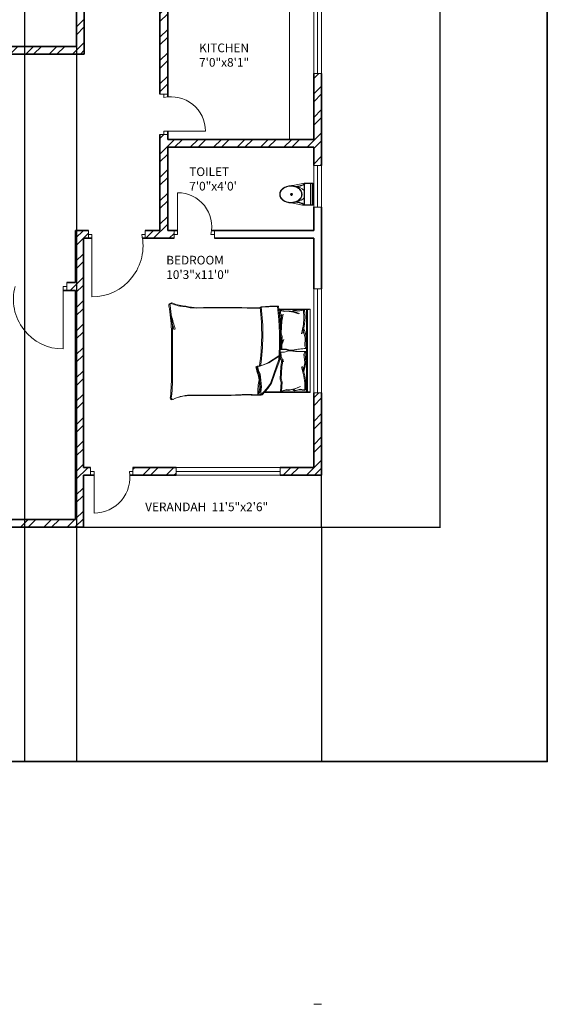
# Model space of a CAD drawing. Units: inches. Extents: x 1885 to 2748, y 783 to 2421.
# Tile 28 of 117: x 2445 to 2748, y 783 to 1350. Entities that reach past the tile are written whole.
import ezdxf

# ---------------------------------------------------------------- set-up
doc = ezdxf.new("R2010")
doc.units = ezdxf.units.IN
for name, color, linetype, lineweight in [('A-ANNO-DIMS', 2, 'Continuous', 18), ('A-ANNO-TTLB', 7, 'Continuous', 35), ('A-AREA-IDEN', 7, 'Continuous', 18), ('A-DOOR', 31, 'Continuous', 18), ('A-FLOR-BALC', 7, 'Continuous', 25), ('A-FLOR-CASE', 9, 'Continuous', 18), ('A-FLOR-FIXT', 8, 'Continuous', 18), ('A-FURN', 8, 'Continuous', 13), ('A-GENL-RVWE', 8, 'Continuous', 13), ('A-GLAZ', 181, 'Continuous', 18), ('A-WALL', 7, 'Continuous', 35)]:
    doc.layers.add(name, color=color, linetype=linetype, lineweight=lineweight)
doc.layers.add('A-WALL-PATT', color=85, linetype='Continuous', lineweight=13, true_color=0x58ba48)
doc.styles.get("Standard").update_dxf_attribs({"font": 'arial.ttf'})
doc.dimstyles.get("Standard").update_dxf_attribs({"dimtxt": 0.18, "dimasz": 0.18, "dimexe": 0.18, "dimexo": 0.0625, "dimgap": 0.09, "dimtad": 0, "dimtih": 1, "dimtoh": 1, "dimdec": 4, "dimzin": 0, "dimdsep": 46, "dimtxsty": 'Standard', "dimcen": 0.09, "dimadec": 0, "dimazin": 0, "dimtfac": 1, "dimtdec": 4, "dimtofl": 0, "dimtmove": 0, "dimatfit": 3, "dimfxl": 1, "dimtolj": 1, "dimtzin": 0, "dimarcsym": 0})

# ---------------------------------------------------------------- blocks, each defined once
blk = doc.blocks.new('A$C31115884')
for p, q in [((283, 498), (223, 498)), ((258, 466), (258, 523)), ((0, 200), (0, 0)), ((520, 200), (0, 200)), ((510, 54), (0, 54)), ((10, 190), (10, 10)), ((510, 190), (10, 190)), ((10, 10), (510, 10)), ((510, 10), (510, 190)), ((520, 0), (520, 200)), ((0, 0), (520, 0))]:
    blk.add_line(p, q)
blk.add_circle((256, 496), 23.6)
for centre, radius, start, end in [((2778, -205), 2807, 165.4549, 171.7133), ((-295, 403), 365, 324.2091, 9.3499), ((-295, 403), 375, 324.2091, 9.3499), ((806, 403), 365, 170.6501, 215.7909), ((3237, 905), 2807, 188.2867, 194.5451), ((384, 406), 293, 190.2774, 224.1564), ((139, 406), 293, 315.8436, 2.6563), ((806, 403), 375, 179.2036, 215.7909)]:
    blk.add_arc(centre, radius, start, end)
blk.add_ellipse((256, 510), major_axis=(0, -261), ratio=0.772727)
blk.add_open_spline([(256, 259), (263, 259), (270, 260), (288, 262), (299, 265), (320, 273), (330, 278), (350, 291), (360, 299), (378, 316), (386, 326), (402, 347), (409, 358), (421, 383), (427, 395), (436, 422), (440, 436), (445, 465), (447, 480), (448, 509), (448, 524), (445, 553), (443, 568), (436, 596), (432, 610), (422, 636), (416, 649), (402, 672), (395, 683), (379, 703), (370, 712), (351, 728), (341, 735), (321, 746), (310, 751), (289, 757), (278, 759), (256, 761), (245, 761), (223, 757), (212, 754), (191, 746), (181, 741), (161, 728), (151, 720), (133, 703), (125, 693), (110, 672), (103, 660), (90, 636), (85, 623), (76, 596), (72, 582), (67, 553), (66, 538), (64, 509), (65, 494), (68, 465), (70, 450), (77, 422), (81, 408), (91, 382), (97, 370), (111, 346), (118, 335), (135, 316), (144, 307), (162, 291), (172, 284), (193, 273), (203, 269), (225, 262), (236, 260), (250, 259), (253, 259), (256, 259)], degree=3, knots=[0, 0, 0, 0, 0.110105, 0.110105, 0.285049, 0.285049, 0.459994, 0.459994, 0.634938, 0.634938, 0.809882, 0.809882, 0.984827, 0.984827, 1.159771, 1.159771, 1.334715, 1.334715, 1.50966, 1.50966, 1.684604, 1.684604, 1.859549, 1.859549, 2.034493, 2.034493, 2.209437, 2.209437, 2.384382, 2.384382, 2.559326, 2.559326, 2.73427, 2.73427, 2.909215, 2.909215, 3.084159, 3.084159, 3.259103, 3.259103, 3.434048, 3.434048, 3.608992, 3.608992, 3.783936, 3.783936, 3.958881, 3.958881, 4.133825, 4.133825, 4.30877, 4.30877, 4.483714, 4.483714, 4.658658, 4.658658, 4.833603, 4.833603, 5.008547, 5.008547, 5.183491, 5.183491, 5.358436, 5.358436, 5.53338, 5.53338, 5.708324, 5.708324, 5.883269, 5.883269, 6.058213, 6.058213, 6.233158, 6.233158, 6.283185, 6.283185, 6.283185, 6.283185])
blk = doc.blocks.new('BED-DOUBLE')
for p, q in [((0, 51.49), (0.64, 51.49)), ((0, 3.47), (0, 51.49)), ((0, 51.26), (26.61, 51.26)), ((0, 51.26), (26.61, 51.26)), ((0.64, 51.49), (27.25, 51.49)), ((0.64, 51.49), (27.25, 51.49)), ((1.54, 3.47), (1.54, 51.26)), ((1.54, 3.47), (1.54, 51.26)), ((2.18, 3.7), (2.18, 51.49)), ((2.18, 3.7), (2.18, 51.49)), ((27.75, 52.87), (24.5, 49.16)), ((27.75, 52.87), (24.5, 49.16)), ((28.39, 53.09), (25.14, 49.39)), ((28.39, 53.09), (25.14, 49.39)), ((29.49, 52.95), (27.75, 52.87, 3.87)), ((29.49, 52.95), (27.75, 52.87, 3.87)), ((28.37, 51.33), (27.75, 52.87)), ((28.37, 51.33), (27.75, 52.87)), ((28.06, 48.23), (28.37, 51.33)), ((28.06, 48.23), (28.37, 51.33)), ((30.13, 53.17), (28.39, 53.09, 3.87)), ((30.13, 53.17), (28.39, 53.09, 3.87)), ((29.01, 51.56), (28.39, 53.09)), ((29.01, 51.56), (28.39, 53.09)), ((28.7, 48.46), (29.01, 51.56)), ((28.7, 48.46), (29.01, 51.56)), ((2.56, 50.11), (2.46, 44.71)), ((2.56, 50.11), (2.46, 44.71)), ((2.46, 44.71), (2.55, 45.71)), ((2.46, 44.71), (2.55, 45.71)), ((2.55, 45.71), (3.07, 41.91)), ((2.55, 45.71), (3.07, 41.91)), ((2.56, 50.11), (5.77, 49.73)), ((2.56, 50.11), (5.77, 49.73)), ((3.2, 50.34), (3.1, 44.94)), ((3.2, 50.34), (3.1, 44.94)), ((3.1, 44.94), (3.19, 45.94)), ((3.1, 44.94), (3.19, 45.94)), ((3.19, 45.94), (3.71, 42.14)), ((3.19, 45.94), (3.71, 42.14)), ((3.2, 50.34), (6.41, 49.96)), ((3.2, 50.34), (6.41, 49.96)), ((8.26, 49.31), (5.58, 48.13)), ((8.26, 49.31), (5.58, 48.13)), ((5.77, 49.73), (8.34, 50.33)), ((5.77, 49.73), (8.34, 50.33)), ((8.9, 49.54), (6.22, 48.36)), ((8.9, 49.54), (6.22, 48.36)), ((6.41, 49.96), (8.98, 50.56)), ((6.41, 49.96), (8.98, 50.56)), ((11.83, 50.11), (8.26, 49.31)), ((11.83, 50.11), (8.26, 49.31)), ((8.34, 50.33), (9.39, 49.81)), ((8.34, 50.33), (9.39, 49.81)), ((12.47, 50.34), (8.9, 49.54)), ((12.47, 50.34), (8.9, 49.54)), ((8.98, 50.56), (10.03, 50.04)), ((8.98, 50.56), (10.03, 50.04)), ((13.44, 49.92), (11.83, 50.11)), ((13.44, 49.92), (11.83, 50.11)), ((14.08, 50.15), (12.47, 50.34)), ((14.08, 50.15), (12.47, 50.34)), ((16.58, 50.7), (13.44, 49.92)), ((16.58, 50.7), (13.44, 49.92)), ((17.22, 50.93), (14.08, 50.15)), ((17.22, 50.93), (14.08, 50.15)), ((16.17, 45.57), (16.58, 50.7)), ((16.17, 45.56), (16.58, 50.7)), ((16.73, 43.6), (16.17, 45.57)), ((16.73, 43.6), (16.17, 45.56)), ((16.81, 45.79), (17.22, 50.93)), ((16.81, 45.79), (17.22, 50.93)), ((17.37, 43.83), (16.81, 45.79)), ((17.37, 43.83), (16.81, 45.79)), ((22.33, 46.22), (20.32, 40.64)), ((22.33, 46.22), (20.32, 40.64)), ((22.97, 46.45), (20.96, 40.87)), ((22.97, 46.45), (20.96, 40.87)), ((24.5, 49.16), (22.33, 46.22)), ((24.5, 49.16), (22.33, 46.22)), ((25.14, 49.39), (22.97, 46.45)), ((25.14, 49.39), (22.97, 46.45)), ((28.37, 44.36), (28.06, 48.23)), ((28.37, 44.36), (28.06, 48.23)), ((29.01, 44.59), (28.7, 48.46)), ((29.01, 44.59), (28.7, 48.46)), ((3.07, 41.91), (4.43, 36.49)), ((3.07, 41.91), (4.43, 36.49)), ((3.71, 42.14), (5.07, 36.72)), ((3.71, 42.14), (5.07, 36.72)), ((16.3, 36.59), (16.73, 43.6)), ((16.3, 36.59), (16.73, 43.6)), ((16.94, 36.82), (17.37, 43.83)), ((16.94, 36.82), (17.37, 43.83)), ((20.32, 40.64), (17.39, 32.3)), ((20.32, 40.64), (17.39, 32.3)), ((20.96, 40.87), (18.03, 32.53)), ((20.96, 40.87), (18.03, 32.53)), ((28.83, 40.95), (28.37, 44.36)), ((28.83, 40.95), (28.37, 44.36)), ((29.76, 38.94), (28.83, 40.95)), ((29.76, 38.94), (28.83, 40.95)), ((29.47, 41.18), (29.01, 44.59)), ((29.47, 41.18), (29.01, 44.59)), ((30.4, 39.17), (29.47, 41.18)), ((30.4, 39.17), (29.47, 41.18)), ((79.89, 15.29), (79.89, 39.9)), ((79.89, 15.29), (79.89, 39.9)), ((3.08, 37.13), (2.54, 34.2)), ((3.08, 37.13), (2.54, 34.2)), ((2.54, 34.2), (2.56, 33.88)), ((2.54, 34.2), (2.56, 33.88)), ((3.68, 39.2), (3.08, 37.13)), ((3.68, 39.2), (3.08, 37.13)), ((3.72, 37.36), (3.18, 34.43)), ((3.72, 37.36), (3.18, 34.43)), ((3.18, 34.43), (3.2, 34.11)), ((3.18, 34.43), (3.2, 34.11)), ((3.2, 34.11), (3.62, 29.68)), ((3.2, 34.11), (3.62, 29.68)), ((4.32, 39.43), (3.72, 37.36)), ((4.32, 39.43), (3.72, 37.36)), ((15.63, 32.56), (16.3, 36.59)), ((15.63, 32.56), (16.3, 36.59)), ((17.38, 30.98), (16.1, 34.05)), ((17.38, 30.98), (16.1, 34.05)), ((16.27, 32.79), (16.94, 36.82)), ((16.27, 32.79), (16.94, 36.82)), ((17.39, 30.26), (23.88, 34.45)), ((17.39, 30.26), (23.88, 34.45)), ((18.03, 30.49), (24.52, 34.68)), ((18.03, 30.49), (24.52, 34.68)), ((23.88, 34.45), (28.37, 36.15)), ((23.88, 34.45), (28.37, 36.15)), ((24.52, 34.68), (29.01, 36.38)), ((24.52, 34.68), (29.01, 36.38)), ((28.37, 36.15), (30.38, 36.46)), ((28.37, 36.15), (30.38, 36.46)), ((29.01, 36.38), (31.02, 36.69)), ((29.01, 36.38), (31.02, 36.69)), ((30.38, 36.46), (29.76, 38.94)), ((30.38, 36.46), (29.76, 38.94)), ((31.02, 36.69), (30.4, 39.17)), ((31.02, 36.69), (30.4, 39.17)), ((79.25, 15.06), (79.25, 39.68)), ((79.25, 15.06), (79.25, 39.68)), ((2.98, 29.45), (2.5, 27.98)), ((2.98, 29.45), (2.5, 27.98)), ((2.56, 33.88), (2.98, 29.45)), ((2.56, 33.88), (2.98, 29.45)), ((3.62, 29.68), (3.13, 28.2)), ((3.62, 29.68), (3.13, 28.2)), ((14.86, 28.36), (17.54, 28.52)), ((14.86, 28.36), (17.54, 28.52)), ((16.74, 30.75), (15.46, 33.82)), ((16.74, 30.75), (15.46, 33.82)), ((16.9, 28.3), (16.74, 30.75)), ((16.9, 28.3), (16.74, 30.75)), ((17.54, 28.52), (17.38, 30.98)), ((17.54, 28.52), (17.38, 30.98)), ((1.87, 25.98), (7.22, 26.56)), ((1.87, 25.98), (7.22, 26.56)), ((2.45, 24.54), (1.87, 25.98)), ((2.45, 24.54), (1.87, 25.98)), ((2.31, 20.09), (2.45, 24.54)), ((2.31, 20.09), (2.45, 24.54)), ((2.5, 27.98), (7.87, 27.73)), ((2.5, 27.98), (7.87, 27.73)), ((2.51, 26.21), (7.86, 26.79)), ((2.51, 26.21), (7.86, 26.79)), ((3.09, 24.76), (2.51, 26.21)), ((3.09, 24.76), (2.51, 26.21)), ((2.95, 20.32), (3.09, 24.76)), ((2.95, 20.32), (3.09, 24.76)), ((3.13, 28.2), (8.51, 27.96)), ((3.13, 28.2), (8.51, 27.96)), ((7.22, 26.56), (10.4, 27.14)), ((7.22, 26.56), (10.4, 27.14)), ((7.86, 26.79), (11.04, 27.37)), ((7.86, 26.79), (11.04, 27.37)), ((7.87, 27.73), (11.08, 27.35)), ((7.87, 27.73), (11.08, 27.35)), ((8.51, 27.96), (11.72, 27.58)), ((8.51, 27.96), (11.72, 27.58)), ((10.4, 27.14), (11.71, 27.14)), ((10.4, 27.14), (11.71, 27.14)), ((11.04, 27.37), (12.35, 27.37)), ((11.04, 27.37), (12.35, 27.37)), ((11.08, 27.35), (12.38, 27.43)), ((11.08, 27.35), (12.38, 27.43)), ((11.71, 27.14), (13.59, 26.56)), ((11.71, 27.14), (13.59, 26.56)), ((11.72, 27.58), (13.02, 27.66)), ((11.72, 27.58), (13.02, 27.66)), ((12.35, 27.37), (14.22, 26.79)), ((12.35, 27.37), (14.22, 26.79)), ((12.38, 27.43), (14.22, 28.13)), ((12.38, 27.43), (14.22, 28.13)), ((13.02, 27.66), (14.86, 28.36)), ((13.02, 27.66), (14.86, 28.36)), ((13.59, 26.56), (16.27, 26.56)), ((13.59, 26.56), (16.27, 26.56)), ((14.22, 28.13), (16.9, 28.3)), ((14.22, 28.13), (16.9, 28.3)), ((14.22, 26.79), (16.91, 26.79)), ((14.22, 26.79), (16.91, 26.79)), ((16.27, 24.1), (15.18, 20.96)), ((16.27, 24.1), (15.18, 20.96)), ((16.91, 24.33), (15.82, 21.19)), ((16.91, 24.33), (15.82, 21.19)), ((16.17, 19.38), (16.58, 24.51)), ((16.17, 19.38), (16.58, 24.51)), ((16.27, 26.56), (16.27, 24.1)), ((16.27, 26.56), (16.27, 24.1)), ((16.81, 19.61), (17.22, 24.74)), ((16.81, 19.61), (17.22, 24.74)), ((16.91, 26.79), (16.91, 24.33)), ((16.91, 26.79), (16.91, 24.33)), ((2.31, 19.77), (2.31, 20.09)), ((2.31, 19.77), (2.31, 20.09)), ((3.03, 16.88), (2.31, 19.77)), ((3.03, 16.88), (2.31, 19.77)), ((2.95, 20), (2.95, 20.32)), ((2.95, 20), (2.95, 20.32)), ((3.67, 17.11), (2.95, 20)), ((3.67, 17.11), (2.95, 20)), ((3.32, 12.11), (4.33, 17.6)), ((3.32, 12.11), (4.33, 17.6)), ((4.39, 15.08), (3.67, 17.11)), ((4.39, 15.08), (3.67, 17.11)), ((3.96, 12.34), (4.97, 17.83)), ((3.96, 12.34), (4.97, 17.83)), ((16.73, 17.42), (16.17, 19.38)), ((16.73, 17.42), (16.17, 19.38)), ((16.3, 10.41), (16.73, 17.42)), ((16.3, 10.41), (16.73, 17.42)), ((17.37, 17.65), (16.81, 19.61)), ((17.37, 17.65), (16.81, 19.61)), ((16.94, 10.64), (17.37, 17.65)), ((16.94, 10.64), (17.37, 17.65)), ((3.75, 14.85), (3.03, 16.88)), ((3.75, 14.85), (3.03, 16.88)), ((3.03, 8.28), (3.32, 12.11)), ((3.03, 8.28), (3.32, 12.11)), ((3.67, 8.51), (3.96, 12.34)), ((3.67, 8.51), (3.96, 12.34)), ((3.01, 8.18), (3.03, 8.28)), ((3.01, 8.18), (3.03, 8.28)), ((3.34, 3.9), (3.01, 8.18)), ((3.34, 3.9), (3.01, 8.18)), ((3.65, 8.41), (3.67, 8.51)), ((3.65, 8.41), (3.67, 8.51)), ((3.98, 4.13), (3.65, 8.41)), ((3.98, 4.13), (3.65, 8.41)), ((8.96, 5.05), (6.21, 6.06)), ((8.96, 5.05), (6.21, 6.06)), ((9.6, 5.28), (6.85, 6.29)), ((9.6, 5.28), (6.85, 6.29)), ((15.63, 6.38), (16.3, 10.41)), ((15.63, 6.38), (16.3, 10.41)), ((16.27, 6.61), (16.94, 10.64)), ((16.27, 6.61), (16.94, 10.64)), ((16.3, 10.41), (16.62, 9.28)), ((16.3, 10.41), (16.62, 9.28)), ((16.62, 9.28), (17.34, 4.18)), ((16.62, 9.28), (17.34, 4.18)), ((16.94, 10.64), (17.26, 9.51)), ((16.94, 10.64), (17.26, 9.51)), ((17.26, 9.51), (17.98, 4.41)), ((17.26, 9.51), (17.98, 4.41)), ((18.11, 3.47), (0, 3.47)), ((18.11, 3.47), (0, 3.47)), ((18.75, 3.7), (0.64, 3.7)), ((18.75, 3.7), (0.64, 3.7)), ((3.32, 3.89), (6.5, 4.47)), ((3.32, 3.89), (6.5, 4.47)), ((3.96, 4.12), (7.14, 4.7)), ((3.96, 4.12), (7.14, 4.7)), ((6.5, 4.47), (9.1, 4.04)), ((6.5, 4.47), (9.1, 4.04)), ((7.14, 4.7), (9.74, 4.27)), ((7.14, 4.7), (9.74, 4.27)), ((12.57, 4.47), (8.96, 5.05)), ((12.57, 4.47), (8.96, 5.05)), ((9.1, 4.04), (10.12, 4.62)), ((9.1, 4.04), (10.12, 4.62)), ((13.21, 4.7), (9.6, 5.28)), ((13.21, 4.7), (9.6, 5.28)), ((9.74, 4.27), (10.75, 4.84)), ((9.74, 4.27), (10.75, 4.84)), ((14.16, 4.76), (12.57, 4.47)), ((14.16, 4.76), (12.57, 4.47)), ((14.8, 4.99), (13.21, 4.7)), ((14.8, 4.99), (13.21, 4.7)), ((17.34, 4.18), (14.16, 4.76)), ((17.34, 4.18), (14.16, 4.76)), ((17.98, 4.41), (14.8, 4.99)), ((17.98, 4.41), (14.8, 4.99))]:
    blk.add_line(p, q)
for centre, radius, start, end in [((-6.65, 51.33), 36.18, 349.8763, 2.5657), ((-6.65, 51.33), 36.18, 349.8763, 2.5657), ((36.32, 182.26), 129.5, 266.9791, 273.8365), ((36.32, 182.26), 129.5, 266.9791, 273.8365), ((-6.01, 51.55), 36.18, 349.8763, 2.5657), ((-6.01, 51.55), 36.18, 349.8763, 2.5657), ((36.96, 182.49), 129.5, 266.9791, 273.8365), ((36.96, 182.49), 129.5, 266.9791, 273.8365), ((67.83, -4508.74), 4561.86, 90.00217, 90.28689), ((67.83, -4508.75), 4561.86, 90.00217, 90.28689), ((68.46, -4508.52), 4561.86, 90.00217, 90.28689), ((68.46, -4508.52), 4561.86, 90.00217, 90.28689), ((68.67, 76.16), 23.07, 267.4714, 296.4681), ((68.67, 76.16), 23.07, 267.4714, 296.4681), ((69.31, 76.38), 23.07, 267.4714, 296.4681), ((69.31, 76.38), 23.07, 267.4714, 296.4681), ((78.87, 54.41), 1.1, 332.6588, 86.02), ((78.87, 54.41), 1.1, 332.6588, 86.02), ((212.28, 41.15), 133.04, 174.4998, 180.6351), ((212.28, 41.15), 133.04, 174.4998, 180.6351), ((79.51, 54.64), 1.1, 332.6588, 86.02), ((79.51, 54.64), 1.1, 332.6588, 86.02), ((212.92, 41.38), 133.04, 174.4998, 180.6351), ((212.92, 41.38), 133.04, 174.4998, 180.6351), ((35.07, 43.74), 6.22, 168.6608, 203.7384), ((35.07, 43.74), 6.22, 168.6608, 203.7384), ((1.49, 31.15), 29.65, 10.6617, 19.8806), ((1.49, 31.15), 29.65, 10.6617, 19.8806), ((35.71, 43.97), 6.22, 168.6608, 203.7384), ((35.71, 43.97), 6.22, 168.6608, 203.7384), ((2.13, 31.38), 29.65, 10.6617, 19.8806), ((2.13, 31.38), 29.65, 10.6617, 19.8806), ((156.32, 17.75), 129.02, 171.7845, 186.9006), ((156.32, 17.75), 129.02, 171.7845, 186.9006), ((156.96, 17.98), 129.02, 171.7845, 186.9006), ((156.96, 17.98), 129.02, 171.7845, 186.9006), ((30.44, 36.64), 0.185, 250.2464, 1.1377), ((30.44, 36.63), 0.185, 250.2464, 1.1377), ((31.08, 36.86), 0.185, 250.2464, 1.1377), ((31.08, 36.86), 0.185, 250.2464, 1.1377), ((182.06, 21.36), 164.97, 176.0865, 186.7821), ((182.06, 21.36), 164.97, 176.0865, 186.7821), ((182.7, 21.59), 164.97, 176.0865, 186.7821), ((182.7, 21.59), 164.97, 176.0865, 186.7821), ((-23.71, -17.22), 106.46, 13.3832, 17.7053), ((-23.71, -17.22), 106.46, 13.3832, 17.7053), ((-23.07, -16.99), 106.46, 13.3832, 17.7053), ((-23.07, -16.99), 106.46, 13.3832, 17.7053), ((200.84, 21.43), 121.76, 182.9958, 189.4091), ((200.84, 21.43), 121.76, 182.9958, 189.4091), ((201.48, 21.65), 121.76, 182.9958, 189.4091), ((201.48, 21.65), 121.76, 182.9958, 189.4091), ((20.1, 85.16), 83.31, 268.7218, 275.604), ((20.1, 85.16), 83.31, 268.7218, 275.604), ((20.74, 85.39), 83.31, 268.7218, 275.604), ((20.74, 85.39), 83.31, 268.7218, 275.604), ((31.18, -167.31), 170.11, 88.4762, 91.0082), ((31.18, -167.31), 170.11, 88.4762, 91.0082), ((31.82, -167.08), 170.11, 88.4762, 91.0082), ((31.82, -167.08), 170.11, 88.4762, 91.0082), ((50.62, 484.82), 482.31, 268.2277, 271.7185), ((50.62, 484.82), 482.31, 268.2277, 271.7185), ((51.26, 485.05), 482.31, 268.2277, 271.7185), ((51.26, 485.05), 482.31, 268.2277, 271.7185), ((64.52, -26.9), 29.63, 76.0648, 88.9113), ((64.52, -26.9), 29.63, 76.0648, 88.9113), ((65.16, -26.67), 29.63, 76.0648, 88.9113), ((65.16, -26.67), 29.63, 76.0648, 88.9113), ((70.28, -21.66), 23.56, 67.9751, 86.652), ((70.28, -21.66), 23.56, 67.9751, 86.652), ((70.92, -21.43), 23.56, 67.9751, 86.652), ((70.92, -21.43), 23.56, 67.9751, 86.652), ((79.72, 1.09), 1.09, 236.1736, 23.4781), ((79.72, 1.09), 1.09, 236.1736, 23.4781), ((80.36, 1.31), 1.09, 236.1736, 23.4781), ((80.36, 1.31), 1.09, 236.1736, 23.4781)]:
    blk.add_arc(centre, radius, start, end)
blk = doc.blocks.new('WIN-60')
for p, q in [((0, 60), (4.5, 60)), ((0, 60), (0, 0)), ((4.5, 60), (2.25, 60)), ((2.25, 60), (2.25, 0)), ((4.5, 0), (4.5, 60)), ((2.25, 0), (0, 0)), ((0, 0), (4.5, 0))]:
    blk.add_line(p, q)
blk = doc.blocks.new('WIN-24')
for p, q in [((0, 4.5), (0, 0)), ((0, 4.5), (24, 4.5)), ((0, 0), (0, 2.25)), ((0, 2.25), (24, 2.25)), ((24, 2.25), (24, 4.5)), ((24, 4.5), (24, 0)), ((24, 0), (0, 0))]:
    blk.add_line(p, q)
blk = doc.blocks.new('WIN-36')
for p, q in [((0, 36), (4.5, 36)), ((0, 36), (0, 0)), ((4.5, 36), (2.25, 36)), ((2.25, 36), (2.25, 0)), ((4.5, 36), (4.5, 0)), ((2.25, 0), (0, 0)), ((0, 0), (4.5, 0))]:
    blk.add_line(p, q)
blk = doc.blocks.new('*D43')
at = {"layer": 'A-ANNO-DIMS', "color": 0, "lineweight": -2, "transparency": 16777216}
for p, q in [((1971.27, 1057.44), (1971.27, 922.48)), ((2618.27, 1057.44), (2618.27, 922.48)), ((1971.45, 922.66), (2294.48, 922.66)), ((2618.09, 922.66), (2295.06, 922.66))]:
    blk.add_line(p, q, dxfattribs=at)
at = {"layer": 'A-ANNO-DIMS', "color": 0, "transparency": 16777216}
for points in [[(1971.45, 922.69), (1971.45, 922.63), (1971.27, 922.66)], [(2618.09, 922.69), (2618.09, 922.63), (2618.27, 922.66)]]:
    blk.add_solid(points, dxfattribs=at)
at = {"layer": 'Defpoints', "color": 0, "transparency": 16777216}
for p in [(1971.27, 1057.51), (2618.27, 1057.51), (2618.27, 922.66)]:
    blk.add_point(p, dxfattribs=at)
at = {"layer": 'A-ANNO-DIMS', "color": 0, "transparency": 16777216, "insert": (2294.77, 922.66), "char_height": 0.18, "attachment_point": 5}
blk.add_mtext('\\A1;647', dxfattribs=at)
blk = doc.blocks.new('*D44')
at = {"layer": 'A-ANNO-DIMS', "color": 0, "lineweight": -2, "transparency": 16777216}
for p, q in [((2618.34, 2352.51), (2686.7, 2352.51)), ((2686.52, 2352.33), (2686.52, 1705.19)), ((2686.52, 1057.69), (2686.52, 1704.82)), ((2618.34, 1057.51), (2686.7, 1057.51))]:
    blk.add_line(p, q, dxfattribs=at)
at = {"layer": 'A-ANNO-DIMS', "color": 0, "transparency": 16777216}
for points in [[(2686.49, 2352.33), (2686.55, 2352.33), (2686.52, 2352.51)], [(2686.49, 1057.69), (2686.55, 1057.69), (2686.52, 1057.51)]]:
    blk.add_solid(points, dxfattribs=at)
at = {"layer": 'Defpoints', "color": 0, "transparency": 16777216}
for p in [(2618.27, 2352.51), (2686.52, 2352.51), (2618.27, 1057.51)]:
    blk.add_point(p, dxfattribs=at)
at = {"layer": 'A-ANNO-DIMS', "color": 0, "transparency": 16777216, "insert": (2686.52, 1705.01), "char_height": 0.18, "attachment_point": 5}
blk.add_mtext('\\A1;1295', dxfattribs=at)
blk = doc.blocks.new('*D55')
at = {"layer": 'A-ANNO-DIMS', "color": 0, "lineweight": -2, "transparency": 16777216}
for p, q in [((2447.27, 1557.94), (2447.27, 922.48)), ((2477.27, 1557.94), (2477.27, 922.48)), ((2447.45, 922.66), (2462.06, 922.66)), ((2477.09, 922.66), (2462.49, 922.66))]:
    blk.add_line(p, q, dxfattribs=at)
at = {"layer": 'A-ANNO-DIMS', "color": 0, "transparency": 16777216}
for points in [[(2447.45, 922.69), (2447.45, 922.63), (2447.27, 922.66)], [(2477.09, 922.69), (2477.09, 922.63), (2477.27, 922.66)]]:
    blk.add_solid(points, dxfattribs=at)
at = {"layer": 'Defpoints', "color": 0, "transparency": 16777216}
for p in [(2447.27, 1558.01), (2477.27, 1558.01), (2477.27, 922.66)]:
    blk.add_point(p, dxfattribs=at)
at = {"layer": 'A-ANNO-DIMS', "color": 0, "transparency": 16777216, "insert": (2462.27, 922.66), "char_height": 0.18, "attachment_point": 5}
blk.add_mtext('\\A1;30', dxfattribs=at)

msp = doc.modelspace()

# ---------------------------------------------------------------- hatches: boundary and pattern name
at = {"layer": 'A-WALL-PATT'}
h = msp.add_hatch(dxfattribs=at)
h.set_pattern_fill('ANSI32', color=256)
h.paths.add_polyline_path([(2007.77, 2318.01), (1980.77, 2318.01), (1980.77, 2281.22), (1985.27, 2281.22), (1985.27, 2313.51), (2007.77, 2313.51), (2007.77, 2315.76)])
h.paths.add_polyline_path([(2094.32, 2318.01), (2067.77, 2318.01), (2067.77, 2313.51), (2094.32, 2313.51), (2094.32, 2315.76)])
h.paths.add_polyline_path([(2131.37, 2315.76), (2131.37, 2318.01), (2131.19, 2318.01), (2112.61, 2318.01), (2112.61, 2313.51), (2117.27, 2313.51), (2117.27, 2255.2), (2121.77, 2255.2), (2121.77, 2313.51), (2131.37, 2313.51)])
h.paths.add_polyline_path([(2190.51, 2318.01), (2155.37, 2318.01), (2155.37, 2313.51), (2169.77, 2313.51), (2169.77, 2229.51), (2121.77, 2229.51), (2121.77, 2233.45), (2119.52, 2233.45), (2117.27, 2233.45), (2117.27, 2201.1), (2121.77, 2201.1), (2121.77, 2225.01), (2169.77, 2225.01), (2169.77, 2165.01), (2306.27, 2165.01), (2306.27, 2066.01), (2310.77, 2066.01), (2344.27, 2066.01), (2486.27, 2066.01), (2486.27, 1886.01), (2483.02, 1886.01), (2483.02, 1881.51), (2486.27, 1881.51), (2486.27, 1880.68), (2490.77, 1880.68), (2490.77, 2070.51), (2344.27, 2070.51), (2310.77, 2070.51), (2310.77, 2165.01), (2310.77, 2173.64), (2308.52, 2173.64), (2306.27, 2173.64), (2306.27, 2169.51), (2174.27, 2169.51), (2174.27, 2313.51), (2190.51, 2313.51), (2190.51, 2315.76)])
h.paths.add_polyline_path([(1985.27, 2221.22), (1980.77, 2221.22), (1980.77, 2165.01), (1992.77, 2165.01), (1992.77, 2141.93), (1997.27, 2141.93), (1997.27, 2165.01), (2117.27, 2165.01), (2117.27, 2163.13), (2121.77, 2163.13), (2121.77, 2172.73), (2119.52, 2172.73), (2117.27, 2172.73), (2117.27, 2169.51), (1985.27, 2169.51)])
h.paths.add_polyline_path([(1997.27, 2105.93), (1992.77, 2105.93), (1992.77, 2070.51), (2016.77, 2070.51), (2016.77, 2059.12), (2019.02, 2059.12), (2021.27, 2059.12), (2021.27, 2070.51), (2117.27, 2070.51), (2117.27, 2022.51), (2114.42, 2022.51), (2114.42, 2018.01), (2123.63, 2018.01), (2123.63, 2020.26), (2123.63, 2022.51), (2121.77, 2022.51), (2121.77, 2142.59), (2119.52, 2142.59), (2117.27, 2142.59), (2117.27, 2075.01), (1997.27, 2075.01)])
h.paths.add_polyline_path([(2092.03, 2020.26), (2092.03, 2022.51), (2021.27, 2022.51), (2021.27, 2035.12), (2016.77, 2035.12), (2016.77, 2018.01), (2016.77, 1978.78), (2021.27, 1978.78), (2021.27, 2018.01), (2092.03, 2018.01)])
h.paths.add_polyline_path([(2260.94, 2022.51), (2153.1, 2022.51), (2153.1, 2020.26), (2153.1, 2018.01), (2155.27, 2018.01), (2155.27, 1886.01), (2107.63, 1886.01), (2107.63, 1881.51), (2182.91, 1881.51), (2182.91, 1883.76), (2182.91, 1886.01), (2159.77, 1886.01), (2159.77, 2018.01), (2260.94, 2018.01), (2260.94, 2020.26)])
h.paths.add_polyline_path([(2047.63, 1883.76), (2047.63, 1886.01), (2021.27, 1886.01), (2021.27, 1918.78), (2019.02, 1918.78), (2016.77, 1918.78), (2016.77, 1881.51), (2047.63, 1881.51)])
h.paths.add_polyline_path([(2306.36, 1883.76), (2306.36, 1886.01), (2296.27, 1886.01), (2296.27, 1982.01), (2316.54, 1982.01), (2316.54, 1984.26), (2316.54, 1986.51), (2296.27, 1986.51), (2296.27, 2022.51), (2289.28, 2022.51), (2289.28, 2018.01), (2291.77, 2018.01), (2291.77, 1886.01), (2242.91, 1886.01), (2242.91, 1881.51), (2306.36, 1881.51)], flags=17)
h.paths.add_polyline_path([(1985.27, 1843.01), (2021.6, 1843.01), (2021.53, 1845.44), (2021.48, 1847.51), (1980.77, 1847.51), (1980.77, 1809.45), (1985.27, 1809.45)])
h.paths.add_polyline_path([(2131.48, 1845.26), (2131.48, 1847.51), (2081.53, 1847.51), (2081.53, 1843.01), (2117.27, 1843.01), (2117.27, 1784.15), (2119.52, 1784.15), (2121.77, 1784.15), (2121.77, 1843.01), (2131.48, 1843.01)])
h.paths.add_polyline_path([(2203.89, 1847.51), (2155.48, 1847.51), (2155.48, 1843.01), (2169.77, 1843.01), (2169.77, 1759.01), (2121.77, 1759.01), (2121.77, 1761.46), (2117.27, 1761.46), (2117.27, 1730.43), (2121.77, 1730.43), (2121.77, 1754.51), (2177.42, 1754.51), (2177.42, 1756.76), (2177.42, 1759.01), (2174.27, 1759.01), (2174.27, 1843.01), (2203.89, 1843.01)])
h.paths.add_polyline_path([(2335.55, 1845.26), (2335.55, 1847.51), (2239.89, 1847.51), (2239.89, 1843.01), (2306.27, 1843.01), (2306.27, 1759.01), (2199.49, 1759.01), (2199.49, 1754.51), (2310.77, 1754.51), (2310.77, 1843.01), (2335.55, 1843.01)])
h.paths.add_polyline_path([(2348.77, 2022.51), (2344.27, 2022.51), (2344.27, 1986.51), (2341.68, 1986.51), (2341.68, 1982.01), (2344.27, 1982.01), (2344.27, 1886.01), (2330.36, 1886.01), (2330.36, 1881.51), (2361.63, 1881.51), (2361.63, 1883.76), (2361.63, 1886.01), (2348.77, 1886.01)], flags=17)
h.paths.add_polyline_path([(2283.25, 2315.76), (2283.25, 2318.01), (2238.51, 2318.01), (2238.51, 2313.51), (2283.25, 2313.51)], flags=17)
h.paths.add_polyline_path([(2363.27, 2348.01), (2388.68, 2348.01), (2388.68, 2350.26), (2388.68, 2352.51), (2358.77, 2352.51), (2358.77, 2348.01), (2358.77, 2318.01), (2344.48, 2318.01), (2344.48, 2313.51), (2358.77, 2313.51), (2358.77, 2229.51), (2310.77, 2229.51), (2310.77, 2231.95), (2306.27, 2231.95), (2306.27, 2205.61), (2310.77, 2205.61), (2310.77, 2225.01), (2358.77, 2225.01), (2358.77, 2211.51), (2452.33, 2211.51), (2452.33, 2213.76), (2452.33, 2216.01), (2363.27, 2216.01), (2363.27, 2318.01)])
h.paths.add_polyline_path([(2310.77, 2313.51), (2320.48, 2313.51), (2320.48, 2315.76), (2320.48, 2318.01), (2302.73, 2318.01), (2302.73, 2313.51), (2306.27, 2313.51), (2306.27, 2251.08), (2310.77, 2251.08)], flags=17)
h.paths.add_polyline_path([(2490.77, 2352.51), (2486.27, 2352.51), (2448.68, 2352.51), (2448.68, 2348.01), (2486.27, 2348.01), (2486.27, 2318.01), (2486.27, 2216.01), (2481.78, 2216.01), (2481.78, 2211.51), (2486.27, 2211.51), (2486.27, 2165.01), (2493.29, 2165.01), (2493.29, 2167.26), (2493.29, 2169.51), (2490.77, 2169.51), (2490.77, 2313.51), (2494.43, 2313.51), (2494.43, 2318.01), (2490.77, 2318.01)])
h.paths.add_polyline_path([(2534.65, 2318.01), (2515.69, 2318.01), (2515.69, 2313.51), (2534.65, 2313.51), (2534.65, 2315.76)])
h.paths.add_polyline_path([(2618.27, 2318.01), (2594.65, 2318.01), (2594.65, 2313.51), (2613.77, 2313.51), (2613.77, 2281.71), (2618.27, 2281.71)])
h.paths.add_polyline_path([(2618.27, 2221.71), (2613.77, 2221.71), (2613.77, 2169.51), (2554.02, 2169.51), (2554.02, 2165.01), (2613.77, 2165.01), (2613.77, 2152.88), (2618.27, 2152.88)])
h.paths.add_polyline_path([(2618.27, 2128.88), (2616.02, 2128.88), (2613.77, 2128.88), (2613.77, 2117.01), (2529.77, 2117.01), (2529.77, 2165.01), (2532.85, 2165.01), (2532.85, 2169.51), (2522.87, 2169.51), (2522.87, 2165.01), (2525.27, 2165.01), (2525.27, 2117.01), (2525.27, 2112.51), (2525.27, 2108.58), (2529.77, 2108.58), (2529.77, 2112.51), (2613.77, 2112.51), (2613.77, 2080.19), (2618.27, 2080.19)])
h.paths.add_polyline_path([(2618.27, 2044.19), (2616.02, 2044.19), (2613.77, 2044.19), (2613.77, 2015.51), (2529.77, 2015.51), (2529.77, 2088.58), (2527.52, 2088.58), (2525.27, 2088.58), (2525.27, 2011.01), (2613.77, 2011.01), (2613.77, 1956.75), (2618.27, 1956.75)])
h.paths.add_polyline_path([(2618.27, 1881.51), (2618.27, 1896.75), (2613.77, 1896.75), (2613.77, 1881.51), (2613.77, 1847.51), (2592.71, 1847.51), (2592.71, 1843.01), (2613.77, 1843.01), (2613.77, 1765.01), (2613.77, 1760.51), (2609.62, 1760.51), (2609.62, 1756.01), (2613.77, 1756.01), (2613.77, 1660.01), (2608.54, 1660.01), (2608.54, 1655.51), (2613.77, 1655.51), (2613.77, 1508.16), (2618.27, 1508.16)])
h.paths.add_polyline_path([(2565.77, 1843.01), (2569, 1843.01), (2569, 1847.51), (2490.77, 1847.51), (2490.77, 1849.7), (2488.52, 1849.7), (2486.27, 1849.7), (2486.27, 1847.51), (2477.27, 1847.51), (2477.27, 1838.51), (2477.27, 1821.49), (2486.27, 1821.49), (2486.27, 1838.51), (2561.27, 1838.51), (2561.27, 1765.01), (2486.27, 1765.01), (2486.27, 1786.16), (2477.27, 1786.16), (2477.27, 1765.01), (2477.27, 1756.01), (2486.27, 1756.01), (2565.77, 1756.01), (2585.62, 1756.01), (2585.62, 1758.26), (2585.62, 1760.51), (2565.77, 1760.51), (2565.77, 1765.01)])
h.paths.add_polyline_path([(2486.27, 1651.01), (2561.27, 1651.01), (2561.27, 1567.01), (2486.27, 1567.01), (2486.27, 1591.32), (2477.27, 1591.32), (2477.27, 1567.01), (2477.27, 1558.01), (2477.27, 1555.44), (2481.77, 1555.44), (2481.77, 1558.01), (2568.65, 1558.01), (2568.65, 1560.26), (2568.65, 1562.51), (2565.77, 1562.51), (2565.77, 1655.51), (2584.54, 1655.51), (2584.54, 1657.76), (2584.54, 1660.01), (2565.77, 1660.01), (2486.27, 1660.01), (2477.27, 1660.01), (2477.27, 1651.01), (2477.27, 1632.99), (2486.27, 1632.99)])
h.paths.add_polyline_path([(2449.97, 1883.76), (2449.97, 1886.01), (2421.63, 1886.01), (2421.63, 1881.51), (2449.97, 1881.51)], flags=17)
h.paths.add_polyline_path([(2447.27, 1847.51), (2395.55, 1847.51), (2395.55, 1843.01), (2442.77, 1843.01), (2442.77, 1809.27), (2447.27, 1809.27)])
h.paths.add_polyline_path([(1985.27, 1749.45), (1980.77, 1749.45), (1980.77, 1694.5), (1985.27, 1694.5), (1985.27, 1694.51), (1986.9, 1694.51), (1986.9, 1697.78), (1986.9, 1699.01), (1985.27, 1699.01)])
h.paths.add_polyline_path([(2152.77, 1699.01), (2121.77, 1699.01), (2121.77, 1703.67), (2119.52, 1703.67), (2117.27, 1703.67), (2117.27, 1699.01), (2009.22, 1699.01), (2009.22, 1694.51), (2148.27, 1694.51), (2148.27, 1692.63), (2152.77, 1692.63)])
h.paths.add_polyline_path([(2016.27, 1694.51), (2011.77, 1694.51), (2011.77, 1558.01), (2040.81, 1558.01), (2040.81, 1560.26), (2040.81, 1562.51), (2016.27, 1562.51)])
h.paths.add_polyline_path([(2152.77, 1663.02), (2150.52, 1663.02), (2148.27, 1663.02), (2148.27, 1562.51), (2100.81, 1562.51), (2100.81, 1558.01), (2165.12, 1558.01), (2165.12, 1560.26), (2165.12, 1562.51), (2152.77, 1562.51), (2152.77, 1610.51), (2224.77, 1610.51), (2224.77, 1607.99), (2229.27, 1607.99), (2229.27, 1615.01), (2152.77, 1615.01)])
h.paths.add_polyline_path([(2238.61, 1560.26), (2238.61, 1562.51), (2229.27, 1562.51), (2229.27, 1588.76), (2227.02, 1588.76), (2224.77, 1588.77), (2224.77, 1562.51), (2189.12, 1562.51), (2189.12, 1558.01), (2238.61, 1558.01)])
h.paths.add_polyline_path([(2336.02, 1560.26), (2336.02, 1562.51), (2310.77, 1562.51), (2310.77, 1656.35), (2308.52, 1656.35), (2306.27, 1656.35), (2306.27, 1562.51), (2286.61, 1562.51), (2286.61, 1558.01), (2336.02, 1558.01)])
h.paths.add_polyline_path([(2447.27, 1690.97), (2445.02, 1690.97), (2442.77, 1690.97), (2442.77, 1687.01), (2306.27, 1687.01), (2306.27, 1680.75), (2310.77, 1680.75), (2310.77, 1682.51), (2442.77, 1682.51), (2442.77, 1562.51), (2396.02, 1562.51), (2396.02, 1558.01), (2447.27, 1558.01)])
h.paths.add_polyline_path([(2447.27, 1749.27), (2445.02, 1749.27), (2442.77, 1749.27), (2442.77, 1717.23), (2447.27, 1717.23)])
h.paths.add_polyline_path([(2044.67, 1521.76), (2044.67, 1524.01), (2007.27, 1524.01), (2007.27, 1503.49), (2009.52, 1503.49), (2011.77, 1503.49), (2011.77, 1519.51), (2044.67, 1519.51)])
h.paths.add_polyline_path([(2177.97, 1521.76), (2177.97, 1524.01), (2104.67, 1524.01), (2104.67, 1519.51), (2145.77, 1519.51), (2145.77, 1387.51), (2143.37, 1387.51), (2143.37, 1383.01), (2251.59, 1383.01), (2251.59, 1385.26), (2251.59, 1387.51), (2150.27, 1387.51), (2150.27, 1519.51), (2177.97, 1519.51)])
h.paths.add_polyline_path([(2298.7, 1524.01), (2237.97, 1524.01), (2237.97, 1519.51), (2282.27, 1519.51), (2282.27, 1387.51), (2279.68, 1387.51), (2279.68, 1383.01), (2286.77, 1383.01), (2286.77, 1419.01), (2312.45, 1419.01), (2312.45, 1421.26), (2312.45, 1423.51), (2286.77, 1423.51), (2286.77, 1519.51), (2298.7, 1519.51), (2298.7, 1521.72)], flags=17)
h.paths.add_polyline_path([(2361.9, 1521.76), (2361.9, 1524.01), (2322.7, 1524.01), (2322.7, 1519.51), (2334.77, 1519.51), (2334.77, 1423.51), (2331.93, 1423.51), (2331.93, 1419.01), (2334.77, 1419.01), (2334.77, 1387.51), (2334.77, 1383.23), (2339.27, 1383.23), (2339.27, 1387.51), (2339.27, 1519.51), (2361.9, 1519.51)], flags=17)
h.paths.add_polyline_path([(2447.27, 1521.76), (2447.27, 1524.01), (2421.9, 1524.01), (2421.9, 1519.51), (2447.27, 1519.51)], flags=17)
h.paths.add_polyline_path([(2481.77, 1529.6), (2479.52, 1529.6), (2477.27, 1529.6), (2477.27, 1524.01), (2474.49, 1524.01), (2474.49, 1519.51), (2477.27, 1519.51), (2477.27, 1334.51), (2296.77, 1334.51), (2296.77, 1240.51), (2160.27, 1240.51), (2160.27, 1180.51), (2112.27, 1180.51), (2112.27, 1207.69), (2110.02, 1207.69), (2107.77, 1207.69), (2107.77, 1171.61), (2112.27, 1171.61), (2112.27, 1176.01), (2160.27, 1176.01), (2160.27, 1092.01), (2144.22, 1092.01), (2144.22, 1087.51), (2189.5, 1087.51), (2189.5, 1089.76), (2189.5, 1092.01), (2164.77, 1092.01), (2164.77, 1236.01), (2296.77, 1236.01), (2296.77, 1231.91), (2301.27, 1231.91), (2301.27, 1330.01), (2481.77, 1330.01), (2481.77, 1387.51)])
h.paths.add_polyline_path([(2618.27, 1448.16), (2613.77, 1448.16), (2613.77, 1382.51), (2529.77, 1382.51), (2525.27, 1382.51), (2525.27, 1307.06), (2529.77, 1307.06), (2529.77, 1378.01), (2613.77, 1378.01), (2613.77, 1354.99), (2618.27, 1354.99)])
h.paths.add_polyline_path([(2618.27, 1318.99), (2613.77, 1318.99), (2613.77, 1281.01), (2529.77, 1281.01), (2529.77, 1283.79), (2527.52, 1283.79), (2525.27, 1283.79), (2525.27, 1228.51), (2516.79, 1228.51), (2516.79, 1224.01), (2533.48, 1224.01), (2533.48, 1226.26), (2533.48, 1228.51), (2529.77, 1228.51), (2529.77, 1276.51), (2613.77, 1276.51), (2613.77, 1266.02), (2618.27, 1266.02)])
h.paths.add_polyline_path([(2618.27, 1134.96), (2613.77, 1134.96), (2613.77, 1092.01), (2594.54, 1092.01), (2594.54, 1087.51), (2618.27, 1087.51)])
h.paths.add_polyline_path([(2534.54, 1092.01), (2509.77, 1092.01), (2509.77, 1087.51), (2534.54, 1087.51), (2534.54, 1089.76)])
h.paths.add_polyline_path([(2481.27, 1224.01), (2484.12, 1224.01), (2484.12, 1226.26), (2484.12, 1228.51), (2476.77, 1228.51), (2476.77, 1198.51), (2471.61, 1198.51), (2471.61, 1194.01), (2476.77, 1194.01), (2476.77, 1062.01), (2436.89, 1062.01), (2436.89, 1057.51), (2476.77, 1057.51), (2481.27, 1057.51), (2481.27, 1062.01), (2481.27, 1087.51), (2485.35, 1087.51), (2485.35, 1089.76), (2485.35, 1092.01), (2481.27, 1092.01), (2481.27, 1117.51)])
h.paths.add_polyline_path([(2439.9, 1198.51), (2349.27, 1198.51), (2349.27, 1194.01), (2349.27, 1180.51), (2301.27, 1180.51), (2301.27, 1201.9), (2299.02, 1201.9), (2296.77, 1201.9), (2296.77, 1172.34), (2299.02, 1172.34), (2301.27, 1172.34), (2301.27, 1176.01), (2349.27, 1176.01), (2349.27, 1092.01), (2334.45, 1092.01), (2334.45, 1087.51), (2349.27, 1087.51), (2349.27, 1057.51), (2353.77, 1057.51), (2376.89, 1057.51), (2376.89, 1059.76), (2376.89, 1062.01), (2353.77, 1062.01), (2353.77, 1087.51), (2353.77, 1180.51), (2353.77, 1194.01), (2439.9, 1194.01), (2439.9, 1196.26)])
h.paths.add_polyline_path([(2270.6, 1089.76), (2270.6, 1092.01), (2249.5, 1092.01), (2249.5, 1087.51), (2270.6, 1087.51)], flags=17)
h.paths.add_polyline_path([(2310.45, 1092.01), (2301.27, 1092.01), (2301.27, 1153.29), (2296.77, 1153.29), (2296.77, 1092.01), (2293.79, 1092.01), (2293.79, 1087.51), (2310.45, 1087.51), (2310.45, 1089.76)], flags=17)
h.paths.add_polyline_path([(2112.27, 1150.33), (2110.02, 1150.33), (2107.77, 1150.33), (2107.77, 1092.01), (2104.47, 1092.01), (2104.47, 1087.51), (2120.22, 1087.51), (2120.22, 1089.76), (2120.22, 1092.01), (2112.27, 1092.01)])
h.paths.add_polyline_path([(2082.17, 1092.01), (2058.14, 1092.01), (2058.14, 1087.51), (2082.17, 1087.51), (2082.17, 1089.76)])
h.paths.add_polyline_path([(1975.77, 1145.64), (1971.27, 1145.64), (1971.27, 1087.51), (1980.77, 1087.51), (1998.14, 1087.51), (1998.14, 1089.76), (1998.14, 1092.01), (1985.27, 1092.01), (1975.77, 1092.01)])
h.paths.add_polyline_path([(2112.27, 1244.38), (2110.02, 1244.38), (2107.77, 1244.38), (2107.77, 1240.51), (1992.27, 1240.51), (1992.27, 1271.01), (1987.77, 1271.01), (1987.77, 1240.51), (1980.77, 1240.51), (1975.77, 1240.51), (1971.27, 1240.51), (1971.27, 1205.64), (1975.77, 1205.64), (1975.77, 1236.01), (2107.77, 1236.01), (2107.77, 1233.44), (2112.27, 1233.44), (2112.27, 1236.01)])
h.paths.add_polyline_path([(2112.27, 1383.01), (2114.78, 1383.01), (2114.78, 1385.26), (2114.78, 1387.51), (2102.48, 1387.51), (2102.48, 1383.01), (2107.77, 1383.01), (2107.77, 1335.01), (2011.77, 1335.01), (2011.77, 1349.94), (2007.27, 1349.94), (2007.27, 1335.01), (1987.77, 1335.01), (1987.77, 1330.51), (1987.77, 1307.01), (1992.27, 1307.01), (1992.27, 1330.51), (2007.27, 1330.51), (2107.77, 1330.51), (2107.77, 1264.71), (2112.27, 1264.71)])
h.paths.add_polyline_path([(2077.86, 1387.51), (2011.77, 1387.51), (2011.77, 1390.04), (2009.52, 1390.04), (2007.27, 1390.04), (2007.27, 1373.94), (2011.77, 1373.94), (2011.77, 1383.01), (2077.86, 1383.01)])
h.paths.add_polyline_path([(2011.77, 1443.49), (2007.27, 1443.49), (2007.27, 1410.25), (2011.77, 1410.25)])

# ---------------------------------------------------------------- linework, layer by layer
at = {"layer": 'A-ANNO-TTLB'}
msp.add_lwpolyline([(1885.16, 2409.17), (2748.2, 2409.17), (2748.2, 922.58), (1885.16, 922.58)], close=True, dxfattribs=at)
at = {"layer": 'A-DOOR'}
for p, q in [((2525.27, 1307.06), (2529.77, 1307.06)), ((2529.77, 1307.06), (2527.52, 1307.06)), ((2527.52, 1307.06), (2527.52, 1305.06)), ((2525.27, 1283.79), (2529.77, 1283.79)), ((2527.52, 1283.79), (2527.52, 1285.79)), ((2527.52, 1285.79), (2551.52, 1285.79)), ((2529.77, 1283.79), (2527.52, 1283.79)), ((2535.48, 1226.26), (2535.48, 1250.26)), ((2484.12, 1228.51), (2484.12, 1224.01)), ((2484.12, 1224.01), (2484.12, 1226.26)), ((2484.12, 1226.26), (2486.12, 1226.26)), ((2486.12, 1226.26), (2486.12, 1190.26)), ((2516.79, 1226.26), (2514.79, 1226.26)), ((2516.79, 1228.51), (2516.79, 1224.01)), ((2516.79, 1224.01), (2516.79, 1226.26)), ((2533.48, 1228.51), (2533.48, 1224.01)), ((2533.48, 1224.01), (2533.48, 1226.26)), ((2533.48, 1226.26), (2535.48, 1226.26)), ((2556.67, 1226.26), (2554.67, 1226.26)), ((2556.67, 1228.51), (2556.67, 1224.01)), ((2556.67, 1224.01), (2556.67, 1226.26)), ((2471.61, 1198.51), (2471.61, 1194.01)), ((2471.61, 1196.26), (2469.61, 1196.26)), ((2469.61, 1196.26), (2469.61, 1160.26)), ((2471.61, 1194.01), (2471.61, 1196.26)), ((2485.35, 1092.01), (2485.35, 1087.51)), ((2485.35, 1087.51), (2485.35, 1089.76)), ((2485.35, 1089.76), (2487.35, 1089.76)), ((2487.35, 1089.76), (2487.35, 1065.76)), ((2509.77, 1089.76), (2507.77, 1089.76)), ((2509.77, 1092.01), (2509.77, 1087.51)), ((2509.77, 1087.51), (2509.77, 1089.76))]:
    msp.add_line(p, q, dxfattribs=at)
for centre, radius, start, end in [((2531.78, 1285.79), 19.74, 0, 102.4614), ((2535.48, 1230.59), 19.67, 347.2851, 90), ((2486.12, 1219.68), 29.42, 270, 12.92), ((2469.61, 1188.92), 28.67, 165.175, 270), ((2487.35, 1086.44), 20.68, 270, 9.24)]:
    msp.add_arc(centre, radius, start, end, dxfattribs=at)
at = {"layer": 'A-FLOR-BALC'}
for p, q in [((2618.27, 1057.51), (2618.27, 1087.51)), ((2481.27, 1057.51), (2618.27, 1057.51))]:
    msp.add_line(p, q, dxfattribs=at)
at = {"layer": 'A-FLOR-CASE'}
msp.add_line((2599.89, 1364.58), (2599.89, 1281.01), dxfattribs=at)
at = {"layer": 'A-GENL-RVWE'}
msp.add_line((2618.27, 782.74), (2613.77, 782.74), dxfattribs=at)
at = {"layer": 'A-WALL'}
for p, q in [((2477.27, 1519.51), (2477.27, 1334.51)), ((2481.77, 1330.01), (2481.77, 1387.51)), ((2525.27, 1307.06), (2525.27, 1382.51)), ((2529.77, 1378.01), (2529.77, 1305.42)), ((2477.27, 1334.51), (2296.77, 1334.51)), ((2301.27, 1330.01), (2481.77, 1330.01)), ((2613.77, 1281.01), (2613.77, 1318.99)), ((2618.27, 1318.99), (2618.27, 1266.02)), ((2525.27, 1228.51), (2525.27, 1283.79)), ((2529.77, 1285.79), (2529.77, 1281.01)), ((2529.77, 1281.01), (2613.77, 1281.01)), ((2529.77, 1276.51), (2613.77, 1276.51)), ((2529.77, 1276.51), (2529.77, 1228.51)), ((2613.77, 1266.02), (2613.77, 1276.51)), ((2613.77, 1228.51), (2613.77, 1242.02)), ((2618.27, 1242.02), (2618.27, 1194.96)), ((2476.77, 1228.51), (2476.77, 1198.51)), ((2476.77, 1224.01), (2476.77, 1228.51)), ((2476.77, 1228.51), (2484.12, 1228.51)), ((2516.79, 1228.51), (2525.27, 1228.51)), ((2529.77, 1228.51), (2535.48, 1228.51)), ((2555.04, 1228.51), (2613.77, 1228.51)), ((2481.27, 1224.01), (2481.27, 1117.51)), ((2486.12, 1224.01), (2481.27, 1224.01)), ((2533.48, 1224.01), (2515.22, 1224.01)), ((2613.77, 1224.01), (2556.67, 1224.01)), ((2613.77, 1194.96), (2613.77, 1224.01)), ((2613.77, 1194.96), (2613.77, 1224.01)), ((2471.61, 1198.51), (2476.77, 1198.51)), ((2476.77, 1194.01), (2469.61, 1194.01)), ((2476.77, 1062.01), (2476.77, 1194.01)), ((2476.77, 1194.01), (2476.77, 1087.51)), ((2613.77, 1092.01), (2613.77, 1134.96)), ((2613.77, 1092.01), (2613.77, 1134.96)), ((2618.27, 1134.96), (2618.27, 1087.51)), ((2481.27, 1117.51), (2481.27, 1092.01)), ((2613.77, 1092.01), (2613.77, 1117.51)), ((2613.77, 1092.01), (2613.77, 1117.51)), ((2481.27, 1092.01), (2485.35, 1092.01)), ((2509.77, 1092.01), (2534.54, 1092.01)), ((2594.54, 1092.01), (2613.77, 1092.01)), ((2476.77, 1062.01), (2476.77, 1087.51)), ((2481.27, 1062.01), (2481.27, 1087.51)), ((2487.35, 1087.51), (2481.27, 1087.51)), ((2534.54, 1087.51), (2508.01, 1087.51)), ((2618.27, 1087.51), (2594.54, 1087.51)), ((2436.89, 1062.01), (2476.77, 1062.01)), ((2481.27, 1062.01), (2481.27, 1057.51)), ((2436.89, 1057.51), (2476.77, 1057.51)), ((2476.77, 1057.51), (2481.27, 1057.51))]:
    msp.add_line(p, q, dxfattribs=at)

# ---------------------------------------------------------------- block references
at = {"layer": 'A-FLOR-FIXT', "xscale": 0.0246256636748975, "yscale": 0.0246256636748975, "zscale": 0.0246256636748975, "rotation": 90}
msp.add_blockref('A$C31115884', (2613.23, 1243.02), dxfattribs=at)
at = {"layer": 'A-FURN', "rotation": 180}
msp.add_blockref('BED-DOUBLE', (2611.8, 1186.74), dxfattribs=at)
at = {"layer": 'A-GLAZ'}
for name, p in [('WIN-36', (2613.77, 1318.99)), ('WIN-60', (2613.77, 1134.97))]:
    msp.add_blockref(name, p, dxfattribs=at)
at = {"layer": 'A-GLAZ', "extrusion": (0, 0, -1), "zscale": -1, "rotation": 90}
for name, p in [('WIN-24', (-2613.78, 1242.02)), ('WIN-60', (-2534.55, 1087.5))]:
    msp.add_blockref(name, p, dxfattribs=at)

# ---------------------------------------------------------------- texts
at = {"layer": 'A-AREA-IDEN', "char_height": 5, "attachment_point": 1}
for s, width, insert in [('KITCHEN\\P7\'0"x8\'1"', 161.7753, (2547.8, 1336.2)), ('TOILET\\P7\'0"x4\'0\'', 133.0668, (2542.14, 1264.87)), ('BEDROOM\\P10\'3"x11\'0"', 117.9772, (2528.91, 1213.92)), ('VERANDAH  11\'5"x2\'6"', 142.58, (2516.78, 1071.81))]:
    msp.add_mtext_dynamic_manual_height_columns(s, width=width, gutter_width=12.5, heights=[0], dxfattribs=dict(at, insert=insert))

# ---------------------------------------------------------------- dimensions: what is measured, and where the dimension line sits
at = {"layer": 'A-ANNO-DIMS'}
dim = msp.add_linear_dim(base=(2686.52, 2352.51), p1=(2618.27, 1057.51), p2=(2618.27, 2352.51), angle=90, dimstyle='Standard', override={"dimdec": 0, "dimlfac": 1, "dimrnd": 0, "dimzin": 0, "dimdsep": 46, "dimlunit": 2}, dxfattribs=at)
dim.commit()
dim.dimension.update_dxf_attribs({"geometry": '*D44', "text_midpoint": (2686.52, 1705.01)})
for base, p1, p2, picture, middle in [((2477.27, 922.66), (2447.27, 1558.01), (2477.27, 1558.01), '*D55', (2462.27, 922.66)), ((2618.27, 922.66), (1971.27, 1057.51), (2618.27, 1057.51), '*D43', (2294.77, 922.66))]:
    dim = msp.add_linear_dim(base=base, p1=p1, p2=p2, dimstyle='Standard', override={"dimdec": 0, "dimlfac": 1, "dimrnd": 0, "dimzin": 0, "dimdsep": 46, "dimlunit": 2}, dxfattribs=at)
    dim.commit()
    dim.dimension.update_dxf_attribs({"geometry": picture, "text_midpoint": middle})

doc.saveas('drawing.dxf')
